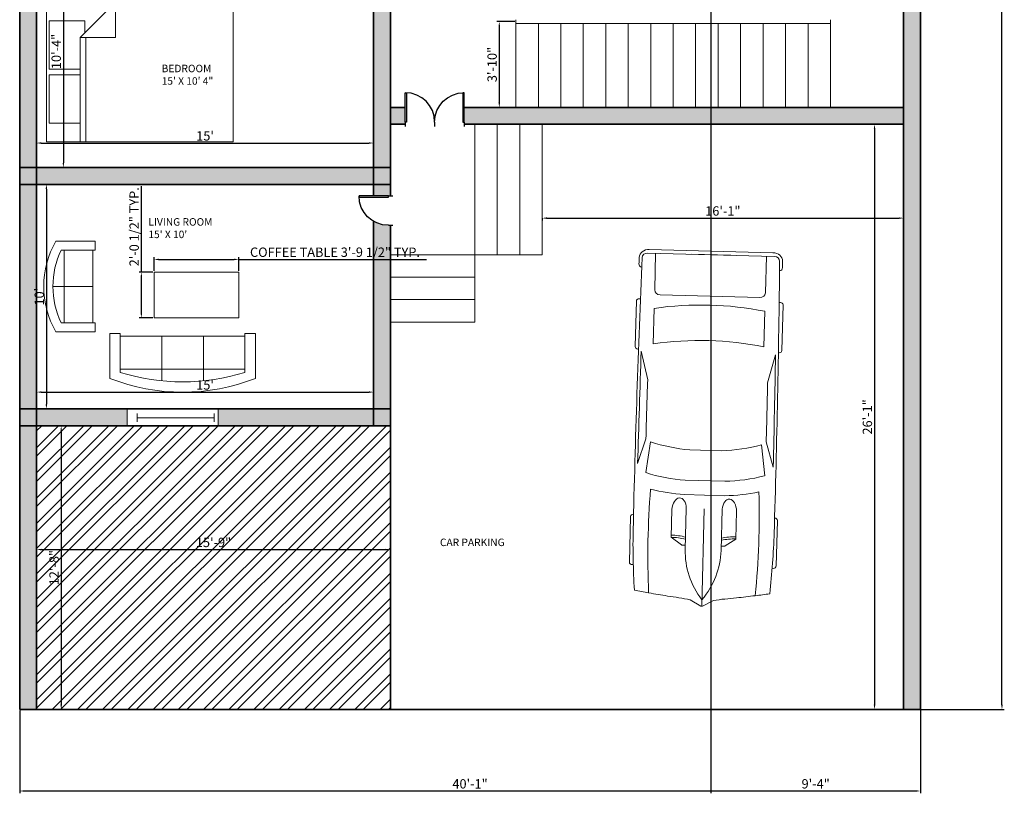
# Model space of a CAD drawing. Units: millimetres. Extents: x 2936 to 3516, y 349 to 1320.
# Tile 1 of 5: x 2990 to 3516, y 349 to 763. Entities that reach past the tile are written whole.
import ezdxf

# ---------------------------------------------------------------- set-up
doc = ezdxf.new("R2010")
doc.units = ezdxf.units.MM
for name, color, linetype, lineweight in [('A-ANNO-DIMS', 3, 'Continuous', 13), ('A-AREA-IDEN', 190, 'Continuous', 18), ('A-FLOR-PATT', 252, 'Continuous', 13), ('A-SITE-VEHI', 140, 'Continuous', 13), ('A-WALL-PATT', 50, 'Continuous', 13), ('doors', 10, 'Continuous', 25), ('furniture', 140, 'Continuous', 18), ('staircase', 170, 'Continuous', 18), ('walls', 50, 'Continuous', 35), ('windows', 30, 'Continuous', 18)]:
    doc.layers.add(name, color=color, linetype=linetype, lineweight=lineweight)
doc.styles.get("Standard").update_dxf_attribs({"font": 'arial.ttf'})
doc.dimstyles.new('ISO-25', dxfattribs={"dimtxt": 5, "dimasz": 2.5, "dimexe": 1.25, "dimexo": 0.625, "dimtad": 1, "dimdec": 0, "dimlunit": 3, "dimtxsty": 'Standard', "dimcen": 2.5, "dimadec": 0, "dimazin": 0, "dimtfac": 1, "dimtdec": 0, "dimtmove": 0, "dimatfit": 3, "dimfxl": 1, "dimarcsym": 0})

# ---------------------------------------------------------------- blocks, each defined once
blk = doc.blocks.new('*U2')
for p, q in [((0, 0), (0, -6)), ((40, 0), (40, -6))]:
    blk.add_line(p, q)
blk.add_lwpolyline([(0, 0), (0, 40), (1.75, 40), (1.75, 0)], close=True)
blk.add_arc((0, 0), 40, 0, 90)
blk = doc.blocks.new('*U4')
for p, q in [((0, 4), (0, 0)), ((0, 2), (36, 2)), ((36, 4), (36, 0))]:
    blk.add_line(p, q)
blk = doc.blocks.new('Bed - Queen')
for p, q in [((0, -80.00003), (0, 0)), ((0, 0), (59.99999, 0)), ((59.99999, 0), (59.99999, -80.00003)), ((7.99999, -1.2), (28.79998, -1.2)), ((7.99999, -14.4), (7.99999, -1.2)), ((28.79998, -1.2), (28.79998, -14.4)), ((31.19999, -1.2), (51.99999, -1.2)), ((31.19999, -14.4), (31.19999, -1.2)), ((51.99999, -1.2), (51.99999, -16.4)), ((0, -14.4), (44.8, -14.4)), ((44.8, -16.8), (0, -16.8)), ((59.99999, -29.6), (44.8, -14.4)), ((44.8, -14.4), (44.8, -29.6)), ((51.99999, -16.4), (46.79936, -16.4)), ((44.8, -29.6), (59.99999, -29.6)), ((59.99999, -80.00003), (0, -80.00003))]:
    blk.add_line(p, q)
blk = doc.blocks.new('Sofa - Roundback 7 ft.')
for p, q in [((-12.00002, -32.4421), (-12.00003, -6.5971)), ((11.99997, -32.4421), (11.99998, -6.5971)), ((-36.000027, -34), (-36.000027, -11.4696)), ((-35.999844, -13.3819), (35.9998, -13.3819)), ((35.99998, -34), (35.99998, -11.4696)), ((-36.000027, -32.4421), (35.99998, -32.4421))]:
    blk.add_line(p, q)
for points in [[(-36.000027, -34), (-42.000027, -34), (-42.000027, -8)], [(41.99998, -8), (41.99998, -34), (35.99998, -34)]]:
    blk.add_lwpolyline(points)
for centre, radius, start, end in [((0, -114.25), 114.25, 68.43141, 111.5686), ((-0.00001, -127.1968), 121.1968, 72.72033, 107.2797)]:
    blk.add_arc(centre, radius, start, end)
blk = doc.blocks.new('Sofa - Roundback Loveseat 5 ft.')
for p, q in [((0, -32.44198), (0, -5.99998)), ((-24, -33.99998), (-24, -11.46958)), ((24.00004, -33.99998), (24.00004, -11.46958)), ((-23.9998, -13.38178), (23.99986, -13.38178)), ((-24, -32.44198), (24.00004, -32.44198))]:
    blk.add_line(p, q)
for points in [[(-24, -33.99998), (-30, -33.99998), (-30, -7.99998)], [(30.00004, -7.99998), (30.00004, -33.99998), (24.00004, -33.99998)]]:
    blk.add_lwpolyline(points)
for centre, radius, start, end in [((0, -60.24998), 60.24998, 60.13715, 119.8628), ((0, -61.38438), 55.38444, 64.32083, 115.6792)]:
    blk.add_arc(centre, radius, start, end)
blk = doc.blocks.new('*U14')
for p, q in [((21.1, 37.41), (21.1, 36.83)), ((46.55, 38.89), (22.35, 38.89)), ((47.8, 37.39), (47.8, 37.41)), ((135.45, 37.07), (135.45, 37.41)), ((136.7, 38.89), (160.9, 38.89)), ((162.15, 37.41), (162.15, 36.77)), ((70.03, 31.54), (86.41, 29.35)), ((87.99, 31.87), (74.76, 35.92)), ((134.31, 35.6), (119.29, 31.78)), ((186.47, -33.5), (186.47, 33.5)), ((188.4, -32.76), (188.4, 32.76)), ((138.42, 29.35), (157.25, 29.35)), ((164.52, 26.39), (164.52, -26.39)), ((186.47, 29.35), (167.01, 29.35)), ((32.27, 11.63), (36.13, 17.17)), ((36.13, 17.17), (50.94, 17.17)), ((32.12, 9.51), (32.12, 11.15)), ((58.92, -10.77), (58.92, 10.77)), ((66.55, -10.53), (66.55, 10.53)), ((186.47, -10.53), (186.47, 10.53)), ((3.27, 6.13), (0.1, 0.41)), ((29.77, 9.51), (51.68, 9.51)), ((82.74, 8.5), (82.74, -8.5)), ((0, 0), (51.68, 0)), ((0.1, -0.41), (3.27, -6.13)), ((29.77, -9.51), (51.68, -9.51)), ((32.12, -9.51), (32.12, -11.15)), ((32.27, -11.63), (36.13, -17.17)), ((36.13, -17.17), (50.94, -17.17)), ((86.41, -29.35), (70.03, -31.54)), ((157.25, -29.35), (138.42, -29.35)), ((167.01, -29.35), (186.47, -29.35)), ((87.99, -31.87), (74.76, -35.92)), ((134.31, -35.6), (119.29, -31.78)), ((21.1, -37.41), (21.1, -36.83)), ((46.55, -38.89), (22.35, -38.89)), ((47.8, -37.39), (47.8, -37.41)), ((135.45, -37.07), (135.45, -37.41)), ((136.7, -38.89), (160.9, -38.89)), ((162.15, -37.41), (162.15, -36.77))]:
    blk.add_line(p, q)
for centre, major_axis, ratio, start_param, end_param in [((41.19, -490.86), (0, 528.23), 0.842304, 0.00281, 0.075598), ((22.35, 37.41), (0, -1.48), 0.842304, 3.141593, 4.712389), ((64.48, -10555.62), (0, 10593.03), 0.842304, -0.013397, 0.002797), ((46.55, 37.41), (0, 1.48), 0.842304, -1.570796, 0), ((136.7, 37.41), (0, -1.48), 0.842304, 3.141593, 4.712389), ((160.9, 37.41), (0, 1.48), 0.842304, -1.570796, 0), ((180.63, 35.84), (0, 2.22), 0.842304, -0.013017, 1.249894), ((64.48, -10556.36), (0, 10595.31), 0.842304, -0.013397, -0.013017), ((183.98, 32.76), (0, -5.25), 0.842304, 1.570796, 3.128196), ((266.03, -27.52), (0, 313.31), 0.842304, 1.367076, 1.39176), ((135.29, 5.39), (0, 81.77), 0.842304, 1.245306, 1.50788), ((64.48, -10555.62), (0, -10591.55), 0.842304, 3.133765, 3.140441), ((95.79, -3666.35), (0, -3698.24), 0.842304, 3.134049, 3.144098), ((183.98, 33.5), (0, -2.96), 0.842304, 1.570796, 3.128196), ((259.18, -27.52), (0, -305.3), 0.842304, 4.528606, 4.561838), ((37.47, -593.96), (0, -623.33), 0.842304, 3.096046, 3.200911), ((134.4, 5.39), (0, -89.78), 0.842304, 4.449482, 4.652344), ((149.6, 2.8), (0, -79.58), 0.842304, 4.372215, 4.640744), ((17.08, 0), (0, 147.02), 0.842304, 4.511394, 4.913384), ((35.91, 0), (0, 147.02), 0.842304, 4.511394, 4.913384), ((167.01, 26.39), (0, 2.96), 0.842304, 0, 1.570796), ((-204.49, 52.4), (0, -250.96), 0.842304, 1.385369, 1.434372), ((13.04, 17.01), (0, 27.42), 0.842304, 4.435146, 4.718221), ((14.2, 17.01), (0, 27.42), 0.842304, 4.435146, 4.718221), ((50.79, 13.34), (6.34, -0.36), 0.603834, -1.395552, 1.581315), ((32.75, 11.15), (0, 0.74), 0.842304, 0.879714, 1.570796), ((29.77, -46.66), (0, 56.17), 0.842304, 0, 0.590319), ((0.62, 0), (0, -0.74), 0.842304, 4.131459, 5.293319), ((29.77, 46.66), (0, 56.17), 0.842304, 2.551274, 3.141593), ((-204.49, -52.4), (0, 250.96), 0.842304, -1.434372, -1.385369), ((13.04, -17.01), (0, -27.42), 0.842304, 1.564964, 1.848039), ((14.2, -17.01), (0, -27.42), 0.842304, 1.564964, 1.848039), ((149.6, -2.8), (0, -79.58), 0.842304, -1.499151, -1.230623), ((32.75, -11.15), (0, -0.74), 0.842304, 4.712389, 5.403472), ((134.4, -5.39), (0, -89.78), 0.842304, -1.510751, -1.307889), ((135.29, -5.39), (0, -81.77), 0.842304, -1.50788, -1.245306), ((259.18, 27.52), (0, 305.3), 0.842304, 1.721348, 1.754579), ((266.03, 27.52), (0, 313.31), 0.842304, 1.749832, 1.774517), ((37.47, 593.96), (0, -623.33), 0.842304, -0.059319, 0.045547), ((167.01, -26.39), (0, -2.96), 0.842304, 4.712389, 6.283185), ((41.19, 490.86), (0, -528.23), 0.842304, -0.075598, -0.00281), ((64.48, 10555.62), (0, 10593.03), 0.842304, 3.138796, 3.15499), ((64.48, 10555.62), (0, -10591.55), 0.842304, 0.001152, 0.007828), ((95.79, 3666.35), (0, -3698.24), 0.842304, -0.002505, 0.007544), ((183.98, -33.5), (0, 2.96), 0.842304, 3.15499, 4.712389), ((183.98, -32.76), (0, -5.25), 0.842304, 0.013397, 1.570796), ((22.35, -37.41), (0, 1.48), 0.842304, 1.570796, 3.141593), ((46.55, -37.41), (0, -1.48), 0.842304, 0, 1.570796), ((136.7, -37.41), (0, -1.48), 0.842304, -1.570796, 0), ((160.9, -37.41), (0, 1.48), 0.842304, 3.141593, 4.712389), ((180.63, -35.84), (0, -2.22), 0.842304, -1.249894, 0.013017), ((64.48, 10556.36), (0, 10595.31), 0.842304, 3.15461, 3.15499)]:
    blk.add_ellipse(centre, major_axis=major_axis, ratio=ratio, start_param=start_param, end_param=end_param)
at = {"extrusion": (0, 0, -1)}
blk.add_ellipse((50.79, -13.34), major_axis=(6.34, 0.36), ratio=0.603834, start_param=-1.395552, end_param=1.581315, dxfattribs=at)
blk = doc.blocks.new('*D28')
at = {"layer": 'A-ANNO-DIMS', "color": 0, "lineweight": -2, "transparency": 16777216}
for p, q in [((3003.81, 807.86), (3014.77, 807.86)), ((3013.52, 805.36), (3013.52, 686.36)), ((3003.81, 683.86), (3014.77, 683.86))]:
    blk.add_line(p, q, dxfattribs=at)
at = {"layer": 'A-ANNO-DIMS', "color": 0, "transparency": 16777216}
for points in [[(3013.11, 805.36), (3013.94, 805.36), (3013.52, 807.86)], [(3013.11, 686.36), (3013.94, 686.36), (3013.52, 683.86)]]:
    blk.add_solid(points, dxfattribs=at)
at = {"layer": 'Defpoints', "color": 0, "transparency": 16777216}
for p in [(3003.19, 807.86), (3003.19, 683.86), (3013.52, 683.86)]:
    blk.add_point(p, dxfattribs=at)
at = {"layer": 'A-ANNO-DIMS', "color": 0, "transparency": 16777216, "insert": (3010.34, 745.86), "char_height": 5, "attachment_point": 5, "rotation": 90}
blk.add_mtext('10\'-4"', dxfattribs=at)
blk = doc.blocks.new('*D29')
at = {"layer": 'A-ANNO-DIMS', "color": 0, "lineweight": -2, "transparency": 16777216}
for p, q in [((2999.19, 690.88), (2999.19, 698.2)), ((3001.69, 696.95), (3176.69, 696.95)), ((3179.19, 690.88), (3179.19, 698.2))]:
    blk.add_line(p, q, dxfattribs=at)
at = {"layer": 'A-ANNO-DIMS', "color": 0, "transparency": 16777216}
for points in [[(3001.69, 697.37), (3001.69, 696.54), (2999.19, 696.95)], [(3176.69, 697.37), (3176.69, 696.54), (3179.19, 696.95)]]:
    blk.add_solid(points, dxfattribs=at)
at = {"layer": 'Defpoints', "color": 0, "transparency": 16777216}
for p in [(3179.19, 696.95), (2999.19, 690.26), (3179.19, 690.26)]:
    blk.add_point(p, dxfattribs=at)
at = {"layer": 'A-ANNO-DIMS', "color": 0, "transparency": 16777216, "insert": (3089.19, 700.13), "char_height": 5, "attachment_point": 5}
blk.add_mtext("15'", dxfattribs=at)
blk = doc.blocks.new('*D30')
at = {"layer": 'A-ANNO-DIMS', "color": 0, "lineweight": -2, "transparency": 16777216}
for p, q in [((3006.73, 674.86), (3003.21, 674.86)), ((3004.46, 672.36), (3004.46, 557.36)), ((3006.73, 554.86), (3003.21, 554.86))]:
    blk.add_line(p, q, dxfattribs=at)
at = {"layer": 'A-ANNO-DIMS', "color": 0, "transparency": 16777216}
for points in [[(3004.04, 672.36), (3004.88, 672.36), (3004.46, 674.86)], [(3004.04, 557.36), (3004.88, 557.36), (3004.46, 554.86)]]:
    blk.add_solid(points, dxfattribs=at)
at = {"layer": 'Defpoints', "color": 0, "transparency": 16777216}
for p in [(3007.36, 674.86), (3004.46, 554.86), (3007.36, 554.86)]:
    blk.add_point(p, dxfattribs=at)
at = {"layer": 'A-ANNO-DIMS', "color": 0, "transparency": 16777216, "insert": (3001.28, 614.86), "char_height": 5, "attachment_point": 5, "rotation": 90}
blk.add_mtext("10'", dxfattribs=at)
blk = doc.blocks.new('*D31')
at = {"layer": 'A-ANNO-DIMS', "color": 0, "lineweight": -2, "transparency": 16777216}
for p, q in [((2999.19, 562.33), (2999.19, 565.11)), ((3001.69, 563.86), (3176.69, 563.86)), ((3179.19, 562.33), (3179.19, 565.11))]:
    blk.add_line(p, q, dxfattribs=at)
at = {"layer": 'A-ANNO-DIMS', "color": 0, "transparency": 16777216}
for points in [[(3001.69, 564.27), (3001.69, 563.44), (2999.19, 563.86)], [(3176.69, 564.27), (3176.69, 563.44), (3179.19, 563.86)]]:
    blk.add_solid(points, dxfattribs=at)
at = {"layer": 'Defpoints', "color": 0, "transparency": 16777216}
for p in [(3179.19, 563.86), (2999.19, 561.7), (3179.19, 561.7)]:
    blk.add_point(p, dxfattribs=at)
at = {"layer": 'A-ANNO-DIMS', "color": 0, "transparency": 16777216, "insert": (3089.19, 567.03), "char_height": 5, "attachment_point": 5}
blk.add_mtext("15'", dxfattribs=at)
blk = doc.blocks.new('*D32')
at = {"layer": 'A-ANNO-DIMS', "color": 0, "lineweight": -2, "transparency": 16777216}
for p, q in [((3254.54, 761.86), (3245.05, 761.86)), ((3246.3, 759.36), (3246.3, 718.44)), ((3254.54, 715.94), (3245.05, 715.94))]:
    blk.add_line(p, q, dxfattribs=at)
at = {"layer": 'A-ANNO-DIMS', "color": 0, "transparency": 16777216}
for points in [[(3245.88, 759.36), (3246.72, 759.36), (3246.3, 761.86)], [(3245.88, 718.44), (3246.72, 718.44), (3246.3, 715.94)]]:
    blk.add_solid(points, dxfattribs=at)
at = {"layer": 'Defpoints', "color": 0, "transparency": 16777216}
for p in [(3255.17, 761.86), (3246.3, 715.94), (3255.17, 715.94)]:
    blk.add_point(p, dxfattribs=at)
at = {"layer": 'A-ANNO-DIMS', "color": 0, "transparency": 16777216, "insert": (3243.12, 738.9), "char_height": 5, "attachment_point": 5, "rotation": 90}
blk.add_mtext('3\'-10"', dxfattribs=at)
blk = doc.blocks.new('*D33')
at = {"layer": 'A-ANNO-DIMS', "color": 0, "lineweight": -2, "transparency": 16777216}
for p, q in [((3411.99, 706.94), (3447.95, 706.94)), ((3446.7, 704.44), (3446.7, 396.79)), ((3411.99, 394.29), (3447.95, 394.29))]:
    blk.add_line(p, q, dxfattribs=at)
at = {"layer": 'A-ANNO-DIMS', "color": 0, "transparency": 16777216}
for points in [[(3446.28, 704.44), (3447.11, 704.44), (3446.7, 706.94)], [(3446.28, 396.79), (3447.11, 396.79), (3446.7, 394.29)]]:
    blk.add_solid(points, dxfattribs=at)
at = {"layer": 'Defpoints', "color": 0, "transparency": 16777216}
for p in [(3411.37, 706.94), (3411.37, 394.29), (3446.7, 394.29)]:
    blk.add_point(p, dxfattribs=at)
at = {"layer": 'A-ANNO-DIMS', "color": 0, "transparency": 16777216, "insert": (3443.52, 550.61), "char_height": 5, "attachment_point": 5, "rotation": 90}
blk.add_mtext('26\'-1"', dxfattribs=at)
blk = doc.blocks.new('*D34')
at = {"layer": 'A-ANNO-DIMS', "color": 0, "lineweight": -2, "transparency": 16777216}
for p, q in [((3269.2, 656.88), (3269.2, 655.58)), ((3271.7, 656.83), (3459.69, 656.83)), ((3462.19, 656.88), (3462.19, 655.58))]:
    blk.add_line(p, q, dxfattribs=at)
at = {"layer": 'A-ANNO-DIMS', "color": 0, "transparency": 16777216}
for points in [[(3271.7, 657.24), (3271.7, 656.41), (3269.2, 656.83)], [(3459.69, 657.24), (3459.69, 656.41), (3462.19, 656.83)]]:
    blk.add_solid(points, dxfattribs=at)
at = {"layer": 'Defpoints', "color": 0, "transparency": 16777216}
for p in [(3269.2, 657.51), (3462.19, 657.51), (3462.19, 656.83)]:
    blk.add_point(p, dxfattribs=at)
at = {"layer": 'A-ANNO-DIMS', "color": 0, "transparency": 16777216, "insert": (3365.69, 660), "char_height": 5, "attachment_point": 5}
blk.add_mtext('16\'-1"', dxfattribs=at)
blk = doc.blocks.new('*D35')
at = {"layer": 'A-ANNO-DIMS', "color": 0, "lineweight": -2, "transparency": 16777216}
for p, q in [((3012.35, 543.36), (3012.35, 396.79)), ((3012.97, 545.86), (3013.6, 545.86)), ((3012.97, 394.29), (3013.6, 394.29))]:
    blk.add_line(p, q, dxfattribs=at)
at = {"layer": 'A-ANNO-DIMS', "color": 0, "transparency": 16777216}
for points in [[(3011.93, 543.36), (3012.76, 543.36), (3012.35, 545.86)], [(3011.93, 396.79), (3012.76, 396.79), (3012.35, 394.29)]]:
    blk.add_solid(points, dxfattribs=at)
at = {"layer": 'Defpoints', "color": 0, "transparency": 16777216}
for p in [(3012.35, 545.86), (3012.35, 394.29), (3012.35, 394.29)]:
    blk.add_point(p, dxfattribs=at)
at = {"layer": 'A-ANNO-DIMS', "color": 0, "transparency": 16777216, "insert": (3009.17, 470.07), "char_height": 5, "attachment_point": 5, "rotation": 90}
blk.add_mtext('12\'-8"', dxfattribs=at)
blk = doc.blocks.new('*D36')
at = {"layer": 'A-ANNO-DIMS', "color": 0, "lineweight": -2, "transparency": 16777216}
for p, q in [((3188.19, 545.23), (3188.19, 478.47)), ((2999.19, 522.68), (2999.19, 478.47)), ((3001.69, 479.72), (3185.69, 479.72))]:
    blk.add_line(p, q, dxfattribs=at)
at = {"layer": 'A-ANNO-DIMS', "color": 0, "transparency": 16777216}
for points in [[(3001.69, 480.14), (3001.69, 479.31), (2999.19, 479.72)], [(3185.69, 480.14), (3185.69, 479.31), (3188.19, 479.72)]]:
    blk.add_solid(points, dxfattribs=at)
at = {"layer": 'Defpoints', "color": 0, "transparency": 16777216}
for p in [(3188.19, 545.86), (2999.19, 523.31), (3188.19, 479.72)]:
    blk.add_point(p, dxfattribs=at)
at = {"layer": 'A-ANNO-DIMS', "color": 0, "transparency": 16777216, "insert": (3093.69, 482.9), "char_height": 5, "attachment_point": 5}
blk.add_mtext('15\'-9"', dxfattribs=at)
blk = doc.blocks.new('COFFEE-TABLE-RECT')
blk.add_lwpolyline([(0, 24.44), (45.27, 24.44), (45.27, 0), (0, 0)], close=True)
blk = doc.blocks.new('*D49')
at = {"layer": 'A-ANNO-DIMS', "color": 0, "lineweight": -2, "transparency": 16777216}
for p, q in [((3061.96, 628.58), (3061.96, 636)), ((3064.46, 634.75), (3104.73, 634.75)), ((3107.23, 628.58), (3107.23, 636)), ((3107.23, 634.75), (3207.39, 634.75))]:
    blk.add_line(p, q, dxfattribs=at)
at = {"layer": 'A-ANNO-DIMS', "color": 0, "transparency": 16777216}
for points in [[(3064.46, 635.16), (3064.46, 634.33), (3061.96, 634.75)], [(3104.73, 635.16), (3104.73, 634.33), (3107.23, 634.75)]]:
    blk.add_solid(points, dxfattribs=at)
at = {"layer": 'Defpoints', "color": 0, "transparency": 16777216}
for p in [(3107.23, 634.75), (3061.96, 627.96), (3107.23, 627.96)]:
    blk.add_point(p, dxfattribs=at)
at = {"layer": 'A-ANNO-DIMS', "color": 0, "transparency": 16777216, "insert": (3158.56, 637.96), "char_height": 5, "attachment_point": 5}
blk.add_mtext('COFFEE TABLE 3\'-9 1/2" TYP.', dxfattribs=at)
blk = doc.blocks.new('*D50')
at = {"layer": 'A-ANNO-DIMS', "color": 0, "lineweight": -2, "transparency": 16777216}
for p, q in [((3055.17, 627.96), (3055.17, 673.92)), ((3061.34, 627.96), (3053.92, 627.96)), ((3055.17, 606.02), (3055.17, 625.46)), ((3061.34, 603.52), (3053.92, 603.52))]:
    blk.add_line(p, q, dxfattribs=at)
at = {"layer": 'A-ANNO-DIMS', "color": 0, "transparency": 16777216}
for points in [[(3054.76, 625.46), (3055.59, 625.46), (3055.17, 627.96)], [(3054.76, 606.02), (3055.59, 606.02), (3055.17, 603.52)]]:
    blk.add_solid(points, dxfattribs=at)
at = {"layer": 'Defpoints', "color": 0, "transparency": 16777216}
for p in [(3055.17, 627.96), (3061.96, 627.96), (3061.96, 603.52)]:
    blk.add_point(p, dxfattribs=at)
at = {"layer": 'A-ANNO-DIMS', "color": 0, "transparency": 16777216, "insert": (3051.96, 652.19), "char_height": 5, "attachment_point": 5, "rotation": 90}
blk.add_mtext('2\'-0 1/2" TYP.', dxfattribs=at)
blk = doc.blocks.new('*D55')
at = {"layer": 'A-ANNO-DIMS', "color": 0, "lineweight": -2, "transparency": 16777216}
for p, q in [((2990.19, 393.66), (2990.19, 349.48)), ((3471.19, 393.66), (3471.19, 349.48)), ((2992.69, 350.73), (3468.69, 350.73))]:
    blk.add_line(p, q, dxfattribs=at)
at = {"layer": 'A-ANNO-DIMS', "color": 0, "transparency": 16777216}
for points in [[(2992.69, 351.15), (2992.69, 350.32), (2990.19, 350.73)], [(3468.69, 351.15), (3468.69, 350.32), (3471.19, 350.73)]]:
    blk.add_solid(points, dxfattribs=at)
at = {"layer": 'Defpoints', "color": 0, "transparency": 16777216}
for p in [(2990.19, 394.29), (3471.19, 394.29), (3471.19, 350.73)]:
    blk.add_point(p, dxfattribs=at)
at = {"layer": 'A-ANNO-DIMS', "color": 0, "transparency": 16777216, "insert": (3230.69, 353.91), "char_height": 5, "attachment_point": 5}
blk.add_mtext('40\'-1"', dxfattribs=at)
blk = doc.blocks.new('*D56')
at = {"layer": 'A-ANNO-DIMS', "color": 0, "lineweight": -2, "transparency": 16777216}
for p, q in [((3471.82, 1265.28), (3515.99, 1265.28)), ((3514.74, 396.79), (3514.74, 1262.78)), ((3471.82, 394.29), (3515.99, 394.29))]:
    blk.add_line(p, q, dxfattribs=at)
at = {"layer": 'A-ANNO-DIMS', "color": 0, "transparency": 16777216}
for points in [[(3514.33, 1262.78), (3515.16, 1262.78), (3514.74, 1265.28)], [(3514.33, 396.79), (3515.16, 396.79), (3514.74, 394.29)]]:
    blk.add_solid(points, dxfattribs=at)
at = {"layer": 'Defpoints', "color": 0, "transparency": 16777216}
for p in [(3471.19, 1265.28), (3514.74, 1265.28), (3471.19, 394.29)]:
    blk.add_point(p, dxfattribs=at)
at = {"layer": 'A-ANNO-DIMS', "color": 0, "transparency": 16777216, "insert": (3511.61, 829.78), "char_height": 5, "attachment_point": 5, "rotation": 90}
blk.add_mtext('72\'-7"', dxfattribs=at)
blk = doc.blocks.new('*D58')
at = {"layer": 'A-ANNO-DIMS', "color": 0, "lineweight": -2, "transparency": 16777216}
for p, q in [((3359.33, 1063.66), (3359.33, 349.48)), ((3471.19, 1063.66), (3471.19, 349.48)), ((3361.83, 350.73), (3468.69, 350.73))]:
    blk.add_line(p, q, dxfattribs=at)
at = {"layer": 'A-ANNO-DIMS', "color": 0, "transparency": 16777216}
for points in [[(3361.83, 351.15), (3361.83, 350.32), (3359.33, 350.73)], [(3468.69, 351.15), (3468.69, 350.32), (3471.19, 350.73)]]:
    blk.add_solid(points, dxfattribs=at)
at = {"layer": 'Defpoints', "color": 0, "transparency": 16777216}
for p in [(3359.33, 1064.28), (3471.19, 1064.28), (3471.19, 350.73)]:
    blk.add_point(p, dxfattribs=at)
at = {"layer": 'A-ANNO-DIMS', "color": 0, "transparency": 16777216, "insert": (3415.26, 353.91), "char_height": 5, "attachment_point": 5}
blk.add_mtext('9\'-4"', dxfattribs=at)

msp = doc.modelspace()

# ---------------------------------------------------------------- hatches: boundary and pattern name
at = {"layer": 'A-FLOR-PATT'}
h = msp.add_hatch(dxfattribs=at)
h.set_pattern_fill('ANSI32', color=256)
h.paths.add_polyline_path([(2999.19, 545.86), (2999.19, 394.29), (3188.19, 394.29), (3188.19, 545.86)])
h.paths.add_polyline_path([(3014.37, 459.71), (3014.37, 480), (3004.06, 480), (3004.06, 459.71)], flags=24)
h.paths.add_polyline_path([(3083.33, 477.7), (3103.62, 477.7), (3103.62, 488.01), (3083.33, 488.01)], flags=24)
at = {"layer": 'A-WALL-PATT'}
h = msp.add_hatch(color=256, dxfattribs=at)
h.dxf.hatch_style = 1
h.paths.add_polyline_path([(2999.19, 1256.28), (2990.19, 1256.28), (2990.19, 1160.28), (2999.19, 1160.28)])
h.paths.add_polyline_path([(2999.19, 1265.28), (2990.19, 1265.28), (2990.19, 1256.28), (2999.19, 1256.28)])
h.paths.add_polyline_path([(3024.89, 1265.28), (2999.19, 1265.28), (2999.19, 1256.28), (3024.89, 1256.28)])
h.paths.add_polyline_path([(3074.24, 1160.28), (2999.19, 1160.28), (2999.19, 1151.28), (3072.14, 1151.28), (3072.14, 1152.43, -0.131652)])
h.paths.add_polyline_path([(2999.19, 1160.28), (2990.19, 1160.28), (2990.19, 1151.28), (2999.19, 1151.28)])
h.paths.add_polyline_path([(3123.19, 1256.28), (3114.19, 1256.28), (3114.19, 1160.28), (3123.19, 1160.28)])
h.paths.add_polyline_path([(3123.19, 1160.28), (3114.19, 1160.28), (3114.19, 1151.28), (3123.19, 1151.28)])
h.paths.add_polyline_path([(3114.19, 1160.28), (3087.85, 1160.28), (3087.85, 1152.43), (3087.85, 1151.28), (3114.19, 1151.28)])
h.paths.add_polyline_path([(3114.19, 1265.28), (3068.72, 1265.28), (3068.72, 1256.28), (3114.19, 1256.28)])
h.paths.add_polyline_path([(3123.19, 1265.28), (3114.19, 1265.28), (3114.19, 1256.28), (3123.19, 1256.28)])
h.paths.add_polyline_path([(3143.16, 1265.28), (3123.19, 1265.28), (3123.19, 1256.28), (3143.16, 1256.28)])
h.paths.add_polyline_path([(3214.19, 1265.28), (3187.49, 1265.28), (3187.49, 1256.28), (3214.19, 1256.28)])
h.paths.add_polyline_path([(3214.19, 1160.28), (3140.09, 1160.28, -0.121149), (3141.88, 1153), (3141.88, 1151.28), (3214.19, 1151.28)])
h.paths.add_polyline_path([(3223.19, 1256.28), (3214.19, 1256.28), (3214.19, 1160.28), (3223.19, 1160.28)])
h.paths.add_polyline_path([(3223.19, 1160.28), (3214.19, 1160.28), (3214.19, 1151.28), (3223.19, 1151.28)])
h.paths.add_polyline_path([(3223.19, 1151.28), (3214.19, 1151.28), (3214.19, 1134.28), (3223.19, 1134.28)])
h.paths.add_polyline_path([(3223.19, 1134.28), (3214.19, 1134.28), (3214.19, 1125.28), (3223.19, 1125.28)])
h.paths.add_polyline_path([(3223.19, 1125.28), (3214.19, 1125.28), (3214.19, 1064.28), (3223.19, 1064.28)])
h.paths.add_polyline_path([(3281.06, 1126.52, -0.130008), (3283.12, 1134.28), (3223.19, 1134.28), (3223.19, 1125.28), (3281.06, 1125.28)])
h.paths.add_polyline_path([(3223.19, 1265.28), (3214.19, 1265.28), (3214.19, 1256.28), (3223.19, 1256.28)])
h.paths.add_polyline_path([(3235.61, 1265.28), (3223.19, 1265.28), (3223.19, 1256.28), (3235.61, 1256.28)])
h.paths.add_polyline_path([(3297.19, 1265.28), (3278.85, 1265.28), (3278.85, 1256.28), (3297.19, 1256.28)])
h.paths.add_polyline_path([(3306.19, 1265.28), (3297.19, 1265.28), (3297.19, 1256.28), (3306.19, 1256.28)])
h.paths.add_polyline_path([(3306.19, 1256.28), (3297.19, 1256.28), (3297.19, 1134.28), (3306.19, 1134.28)])
h.paths.add_polyline_path([(3306.19, 1134.28), (3297.19, 1134.28), (3297.19, 1125.28), (3306.19, 1125.28)])
h.paths.add_polyline_path([(3306.19, 1125.28), (3297.19, 1125.28), (3297.19, 1084.87), (3305.61, 1084.87), (3306.19, 1084.87)])
h.paths.add_polyline_path([(3365.17, 1265.28), (3306.19, 1265.28), (3306.19, 1256.28), (3365.17, 1256.28)])
h.paths.add_polyline_path([(3462.19, 1265.28), (3409.24, 1265.28), (3409.24, 1256.28), (3462.19, 1256.28)])
h.paths.add_polyline_path([(3471.19, 1265.28), (3462.19, 1265.28), (3462.19, 1256.28), (3471.19, 1256.28)])
h.paths.add_polyline_path([(3471.19, 1256.28), (3462.19, 1256.28), (3462.19, 1225.41), (3471.19, 1225.41)])
h.paths.add_polyline_path([(3471.19, 1177.19), (3462.19, 1177.19), (3462.19, 1064.28), (3471.19, 1064.28)])
h.paths.add_polyline_path([(3462.19, 1064.28), (3368.33, 1064.28), (3368.33, 1055.28), (3462.19, 1055.28)])
h.paths.add_polyline_path([(3471.19, 1064.28), (3462.19, 1064.28), (3462.19, 1055.28), (3471.19, 1055.28)])
h.paths.add_polyline_path([(3471.19, 1055.28), (3462.19, 1055.28), (3462.19, 969.86), (3471.19, 969.86)])
h.paths.add_polyline_path([(3368.33, 1055.28), (3359.33, 1055.28), (3359.33, 995.28), (3368.33, 995.28)])
h.paths.add_polyline_path([(3368.33, 1064.28), (3359.33, 1064.28), (3359.33, 1055.28), (3368.33, 1055.28)])
h.paths.add_polyline_path([(3359.33, 995.28), (3306.19, 995.28), (3306.19, 986.28), (3359.33, 986.28)])
h.paths.add_polyline_path([(3368.33, 995.28), (3359.33, 995.28), (3359.33, 986.28), (3368.33, 986.28)])
h.paths.add_polyline_path([(3306.19, 995.28), (3297.19, 995.28), (3297.19, 986.28), (3306.19, 986.28)])
h.paths.add_polyline_path([(3306.19, 1011.04), (3298.85, 1011.04), (3297.19, 1011.04), (3297.19, 995.28), (3306.19, 995.28)])
h.paths.add_polyline_path([(3306.19, 1055.28), (3297.19, 1055.28), (3297.19, 1026.75), (3298.85, 1026.75, -0.122211), (3306.19, 1024.93)])
h.paths.add_polyline_path([(3306.19, 1064.28), (3297.19, 1064.28), (3297.19, 1055.28), (3306.19, 1055.28)])
h.paths.add_polyline_path([(3297.19, 1064.28), (3223.19, 1064.28), (3223.19, 1055.28), (3297.19, 1055.28)])
h.paths.add_polyline_path([(3223.19, 1064.28), (3214.19, 1064.28), (3214.19, 1055.28), (3223.19, 1055.28)])
h.paths.add_polyline_path([(3223.19, 1055.28), (3214.19, 1055.28), (3214.19, 1031.96), (3221.18, 1031.96), (3223.19, 1031.96)])
h.paths.add_polyline_path([(3223.19, 1016.25), (3221.18, 1016.25, -0.11578), (3214.19, 1017.89), (3214.19, 995.28), (3223.19, 995.28)])
h.paths.add_polyline_path([(3223.19, 995.28), (3214.19, 995.28), (3214.19, 986.28), (3223.19, 986.28)])
h.paths.add_polyline_path([(3214.19, 995.28), (3061.3, 995.28), (3061.3, 986.28), (3214.19, 986.28)])
h.paths.add_polyline_path([(2999.19, 1151.28), (2990.19, 1151.28), (2990.19, 995.28), (2999.19, 995.28)])
h.paths.add_polyline_path([(2999.19, 986.28), (2990.19, 986.28), (2990.19, 816.86), (2999.19, 816.86)])
h.paths.add_polyline_path([(2999.19, 995.28), (2990.19, 995.28), (2990.19, 986.28), (2999.19, 986.28)])
h.paths.add_polyline_path([(3016.23, 995.28), (2999.19, 995.28), (2999.19, 986.28), (3016.23, 986.28)])
h.paths.add_polyline_path([(2999.19, 807.86), (2990.19, 807.86), (2990.19, 683.86), (2999.19, 683.86)])
h.paths.add_polyline_path([(2999.19, 816.86), (2990.19, 816.86), (2990.19, 807.86), (2999.19, 807.86)])
h.paths.add_polyline_path([(3179.19, 816.86), (2999.19, 816.86), (2999.19, 807.86), (3179.19, 807.86)])
h.paths.add_polyline_path([(3188.19, 780.83), (3187.16, 780.83, -0.133677), (3179.19, 783), (3179.19, 683.86), (3188.19, 683.86)])
h.paths.add_polyline_path([(3188.19, 807.86), (3179.19, 807.86), (3179.19, 796.54), (3187.16, 796.54), (3188.19, 796.54)])
h.paths.add_polyline_path([(3188.19, 816.86), (3179.19, 816.86), (3179.19, 807.86), (3188.19, 807.86)])
h.paths.add_polyline_path([(3196.08, 816.86), (3188.19, 816.86), (3188.19, 807.86), (3196.08, 807.86)])
h.paths.add_polyline_path([(3321.19, 816.86), (3227.5, 816.86), (3227.5, 807.86), (3321.19, 807.86)])
h.paths.add_polyline_path([(3330.19, 867.56), (3321.19, 867.56), (3321.19, 816.86), (3330.19, 816.86)])
h.paths.add_polyline_path([(3330.19, 816.86), (3321.19, 816.86), (3321.19, 807.86), (3330.19, 807.86)])
h.paths.add_polyline_path([(3462.19, 816.86), (3330.19, 816.86), (3330.19, 807.86), (3462.19, 807.86)])
h.paths.add_polyline_path([(3471.19, 960.86), (3462.19, 960.86), (3462.19, 816.86), (3471.19, 816.86)])
h.paths.add_polyline_path([(3471.19, 816.86), (3462.19, 816.86), (3462.19, 807.86), (3471.19, 807.86)])
h.paths.add_polyline_path([(3471.19, 807.86), (3462.19, 807.86), (3462.19, 394.29), (3471.19, 394.29)])
h.paths.add_polyline_path([(3462.19, 715.94), (3227.5, 715.94), (3227.5, 708.13), (3227.5, 706.94), (3462.19, 706.94)])
h.paths.add_polyline_path([(3196.08, 715.94), (3188.19, 715.94), (3188.19, 706.94), (3196.08, 706.94), (3196.08, 708.13)])
h.paths.add_polyline_path([(2999.19, 674.86), (2990.19, 674.86), (2990.19, 554.86), (2999.19, 554.86)])
h.paths.add_polyline_path([(3179.19, 683.86), (2999.19, 683.86), (2999.19, 674.86), (3179.19, 674.86)])
h.paths.add_polyline_path([(2999.19, 683.86), (2990.19, 683.86), (2990.19, 674.86), (2999.19, 674.86)])
h.paths.add_polyline_path([(2999.19, 545.86), (2990.19, 545.86), (2990.19, 394.29), (2999.19, 394.29)])
h.paths.add_polyline_path([(3047.58, 554.86), (2999.19, 554.86), (2999.19, 545.86), (3047.58, 545.86)])
h.paths.add_polyline_path([(2999.19, 554.86), (2990.19, 554.86), (2990.19, 545.86), (2999.19, 545.86)])
h.paths.add_polyline_path([(3179.19, 554.86), (3096.19, 554.86), (3096.19, 545.86), (3179.19, 545.86)])
h.paths.add_polyline_path([(3188.19, 554.86), (3179.19, 554.86), (3179.19, 545.86), (3188.19, 545.86)])
h.paths.add_polyline_path([(3188.19, 652.99), (3187.11, 652.99, -0.132871), (3179.19, 655.13), (3179.19, 554.86), (3188.19, 554.86)])
h.paths.add_polyline_path([(3188.19, 683.86), (3179.19, 683.86), (3179.19, 674.86), (3188.19, 674.86)])
h.paths.add_polyline_path([(3188.19, 674.86), (3179.19, 674.86), (3179.19, 668.7), (3187.11, 668.7), (3188.19, 668.7)])
h.paths.add_polyline_path([(3462.19, 969.86), (3330.19, 969.86), (3330.19, 960.86), (3462.19, 960.86)])
h.paths.add_polyline_path([(3330.19, 969.86), (3321.19, 969.86), (3321.19, 960.86), (3330.19, 960.86)])
h.paths.add_polyline_path([(3330.19, 960.86), (3321.19, 960.86), (3321.19, 927.28), (3330.19, 927.28)])

# ---------------------------------------------------------------- linework, layer by layer
at = {"layer": 'staircase'}
for p, q in [((3255.17, 762.86), (3255.17, 760.86)), ((3423.17, 760.86), (3423.17, 762.86)), ((3255.17, 760.86), (3423.17, 760.86)), ((3255.17, 760.86), (3255.17, 715.94)), ((3267.17, 760.86), (3267.17, 715.94)), ((3279.17, 760.86), (3279.17, 715.94)), ((3291.17, 760.86), (3291.17, 715.94)), ((3303.17, 760.86), (3303.17, 715.94)), ((3315.17, 760.86), (3315.17, 715.94)), ((3327.17, 760.86), (3327.17, 715.94)), ((3339.17, 760.86), (3339.17, 715.94)), ((3351.17, 760.86), (3351.17, 715.94)), ((3363.17, 760.86), (3363.17, 715.94)), ((3375.17, 760.86), (3375.17, 715.94)), ((3387.17, 760.86), (3387.17, 715.94)), ((3399.17, 760.86), (3399.17, 715.94)), ((3411.17, 760.86), (3411.17, 715.94)), ((3423.17, 760.86), (3423.17, 715.94)), ((3423.17, 715.94), (3255.17, 715.94)), ((3233.2, 706.94), (3233.2, 637.29)), ((3245.2, 706.94), (3245.2, 637.29)), ((3257.2, 706.94), (3257.2, 637.29)), ((3269.2, 706.94), (3269.2, 637.29)), ((3233.2, 637.29), (3188.19, 637.29)), ((3233.2, 637.29), (3188.19, 637.29)), ((3233.2, 637.29), (3233.2, 601.29)), ((3233.2, 637.29), (3269.2, 637.29)), ((3233.2, 625.29), (3188.19, 625.29)), ((3233.2, 613.29), (3188.19, 613.29)), ((3233.2, 601.29), (3188.19, 601.29))]:
    msp.add_line(p, q, dxfattribs=at)
at = {"layer": 'walls'}
for p, q in [((2990.19, 1265.28), (2990.19, 394.29)), ((2999.19, 1265.28), (2999.19, 394.29)), ((3462.19, 1265.28), (3462.19, 394.29)), ((3471.19, 1265.28), (3471.19, 394.29)), ((3179.19, 783), (3179.19, 668.7)), ((3188.19, 780.83), (3188.19, 668.7)), ((3196.08, 715.94), (3188.19, 715.94)), ((3462.19, 715.94), (3226.81, 715.94)), ((3423.17, 715.94), (3462.19, 715.94)), ((3196.08, 706.94), (3188.19, 706.94)), ((3462.19, 706.94), (3227.5, 706.94)), ((3188.19, 683.86), (2990.19, 683.86)), ((3188.19, 674.86), (2990.19, 674.86)), ((3179.19, 655.13), (3179.19, 545.86)), ((3188.19, 652.99), (3188.19, 545.86)), ((3188.19, 554.86), (2990.19, 554.86)), ((3188.19, 545.86), (2990.19, 545.86)), ((3188.19, 545.86), (3188.19, 394.29)), ((2990.19, 394.29), (3471.19, 394.29))]:
    msp.add_line(p, q, dxfattribs=at)
at = {"layer": 'windows'}
for p, q in [((3047.58, 554.86), (3047.58, 545.86)), ((3096.19, 554.86), (3096.19, 545.86))]:
    msp.add_line(p, q, dxfattribs=at)

# ---------------------------------------------------------------- block references
at = {"layer": 'A-SITE-VEHI', "xscale": 1.007589495291339, "yscale": 1.007589495291339, "zscale": 1.007589495291339, "rotation": 88.4789872947209}
msp.add_blockref('*U14', (3354.38, 449.44), dxfattribs=at)
at = {"layer": 'doors', "yscale": 0.3927729305520136, "zscale": 0.3927729305520136}
for p, xscale, rotation in [((3196.08, 708.13), 0.3927729305520136, 1.02022929505e-05), ((3227.5, 708.13), -0.3927729305520136, 359.9999897977093), ((3187.11, 668.7), -0.3927729305520136, 90)]:
    msp.add_blockref('*U2', p, dxfattribs=dict(at, xscale=xscale, rotation=rotation))
at = {"layer": 'furniture'}
for name, p, xscale, yscale, zscale, rotation in [('Bed - Queen', (3004.51, 697.53), 1.245124643961403, 1.245124643961403, 1.245124643961403, 90), ('Sofa - Roundback Loveseat 5 ft.', (3003.07, 620.33), 0.8087673324917968, 0.8087673324917968, 0.8087673324917968, 90), ('Sofa - Roundback 7 ft.', (3077.21, 563.81), 0.9243959546179767, 0.9243959546179767, 0.9243959546179767, 180)]:
    msp.add_blockref(name, p, dxfattribs=dict(at, xscale=xscale, yscale=yscale, zscale=zscale, rotation=rotation))
msp.add_blockref('COFFEE-TABLE-RECT', (3061.96, 603.52), dxfattribs=at)
at = {"layer": 'windows', "xscale": 1.142279500402185, "yscale": 1.142279500402185, "zscale": 1.142279500402185}
msp.add_blockref('*U4', (3052.9, 547.91), dxfattribs=at)

# ---------------------------------------------------------------- texts
at = {"layer": 'A-AREA-IDEN', "char_height": 4, "attachment_point": 1}
for s, width, insert in [('BEDROOM \\P15\' X 10\' 4"', 63.6228, (3066.01, 738.78)), ("LIVING ROOM \\P15' X 10' ", 54.9715, (3058.92, 656.81)), ('CAR PARKING', 61.3905, (3214.61, 485.58))]:
    msp.add_mtext_dynamic_manual_height_columns(s, width=width, gutter_width=12.5, heights=[0], dxfattribs=dict(at, insert=insert))

# ---------------------------------------------------------------- dimensions: what is measured, and where the dimension line sits
at = {"layer": 'A-ANNO-DIMS'}
for base, p1, p2, override, picture, middle in [((3514.74, 1265.28), (3471.19, 394.29), (3471.19, 1265.28), {"dimdec": 1, "dimlfac": 1, "dimrnd": 0, "dimzin": 1, "dimdsep": 46, "dimlunit": 4, "dimfrac": 2}, '*D56', (3511.61, 829.78)), ((3013.52, 683.86), (3003.19, 807.86), (3003.19, 683.86), {"dimclrd": 0, "dimclre": 0, "dimclrt": 0}, '*D28', (3010.34, 745.86)), ((3246.3, 715.94), (3255.17, 761.86), (3255.17, 715.94), {"dimclrd": 0, "dimclre": 0, "dimclrt": 0}, '*D32', (3243.12, 738.9)), ((3446.7, 394.29), (3411.37, 706.94), (3411.37, 394.29), {"dimclrd": 0, "dimclre": 0, "dimclrt": 0}, '*D33', (3443.52, 550.61)), ((3004.46, 554.86), (3007.36, 674.86), (3007.36, 554.86), {"dimclrd": 0, "dimclre": 0, "dimclrt": 0}, '*D30', (3001.28, 614.86)), ((3012.35, 394.29), (3012.35, 545.86), (3012.35, 394.29), {"dimclrd": 0, "dimclre": 0, "dimclrt": 0}, '*D35', (3009.17, 470.07))]:
    dim = msp.add_linear_dim(base=base, p1=p1, p2=p2, angle=90, dimstyle='ISO-25', override=override, dxfattribs=at)
    dim.commit()
    dim.dimension.update_dxf_attribs({"geometry": picture, "text_midpoint": middle})
for base, p1, p2, override, picture, middle in [((3471.19, 350.73), (3359.33, 1064.28), (3471.19, 1064.28), {"dimdec": 1, "dimlfac": 1, "dimrnd": 0, "dimzin": 1, "dimdsep": 46, "dimlunit": 4, "dimfrac": 2}, '*D58', (3415.26, 353.91)), ((3179.19, 696.95), (2999.19, 690.26), (3179.19, 690.26), {"dimclrd": 0, "dimclre": 0, "dimclrt": 0}, '*D29', (3089.19, 700.13)), ((3462.19, 656.83), (3269.2, 657.51), (3462.19, 657.51), {"dimclrd": 0, "dimclre": 0, "dimclrt": 0}, '*D34', (3365.69, 660)), ((3179.19, 563.86), (2999.19, 561.7), (3179.19, 561.7), {"dimclrd": 0, "dimclre": 0, "dimclrt": 0}, '*D31', (3089.19, 567.03)), ((3188.19, 479.72), (2999.19, 523.31), (3188.19, 545.86), {"dimclrd": 0, "dimclre": 0, "dimclrt": 0}, '*D36', (3093.69, 482.9)), ((3471.19, 350.73), (2990.19, 394.29), (3471.19, 394.29), {"dimdec": 1, "dimlfac": 1, "dimrnd": 0, "dimzin": 1, "dimdsep": 46, "dimlunit": 4, "dimfrac": 2}, '*D55', (3230.69, 353.91))]:
    dim = msp.add_linear_dim(base=base, p1=p1, p2=p2, dimstyle='ISO-25', override=override, dxfattribs=at)
    dim.commit()
    dim.dimension.update_dxf_attribs({"geometry": picture, "text_midpoint": middle})
dim = msp.add_linear_dim(base=(3055.17, 627.96), p1=(3061.96, 603.52), p2=(3061.96, 627.96), angle=90, text='<> TYP.', dimstyle='ISO-25', override={"dimdec": 1, "dimlfac": 1, "dimrnd": 0, "dimzin": 1, "dimdsep": 46, "dimlunit": 4, "dimfrac": 2}, dxfattribs=at)
dim.commit()
dim.dimension.update_dxf_attribs({"geometry": '*D50', "text_midpoint": (3051.96, 652.19)})
dim = msp.add_linear_dim(base=(3107.23, 634.75), p1=(3061.96, 627.96), p2=(3107.23, 627.96), text='COFFEE TABLE <> TYP.', dimstyle='ISO-25', override={"dimdec": 1, "dimlfac": 1, "dimrnd": 0, "dimzin": 1, "dimdsep": 46, "dimlunit": 4, "dimfrac": 2}, dxfattribs=at)
dim.commit()
dim.dimension.update_dxf_attribs({"geometry": '*D49', "text_midpoint": (3158.56, 637.96)})

doc.saveas('drawing.dxf')
